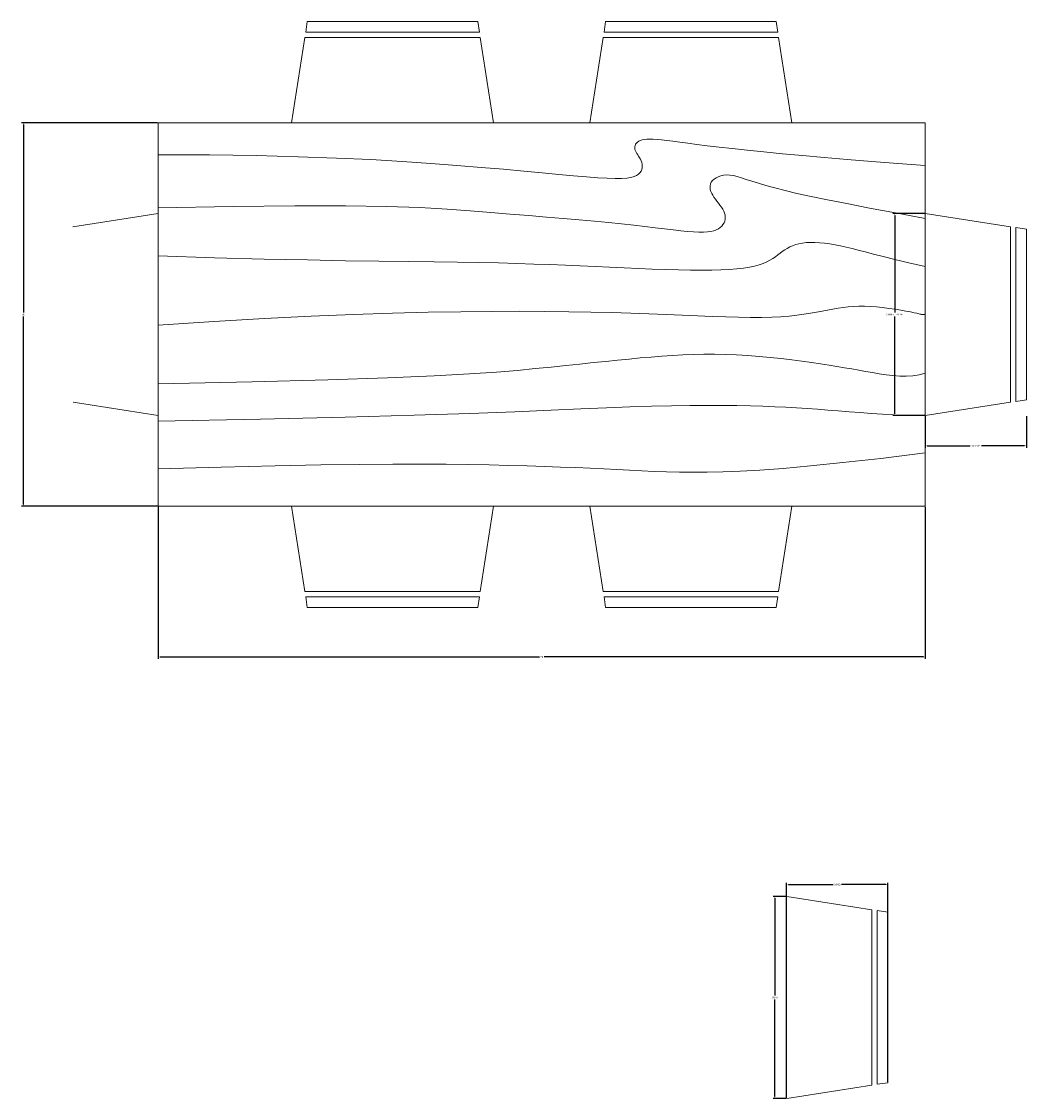
# Model space of a CAD drawing. Units: inches. Extents: x 821 to 2399, y 74 to 823.
# Tile 10 of 13: x 1930 to 2024, y 382 to 483. Entities that reach past the tile are written whole.
import ezdxf

# ---------------------------------------------------------------- set-up
doc = ezdxf.new("R2010")
doc.units = ezdxf.units.IN
doc.header["$MEASUREMENT"] = 0
doc.layers.get('0').update_dxf_attribs({"lineweight": 53})
doc.layers.add('A-ANNO-DIMS', color=2, linetype='Continuous', lineweight=18)
doc.layers.add('A-FURN', color=8, linetype='Continuous', lineweight=18)
doc.styles.get("Standard").update_dxf_attribs({"font": 'arial.ttf'})
doc.dimstyles.get("Standard").update_dxf_attribs({"dimtxt": 0.18, "dimasz": 0.18, "dimexe": 0.18, "dimexo": 0.0625, "dimgap": 0.09, "dimtad": 0, "dimtih": 1, "dimtoh": 1, "dimdec": 4, "dimzin": 0, "dimdsep": 46, "dimtxsty": 'Standard', "dimcen": 0.09, "dimadec": 0, "dimazin": 0, "dimtfac": 1, "dimtdec": 4, "dimtofl": 0, "dimtmove": 0, "dimatfit": 3, "dimfxl": 1, "dimtolj": 1, "dimtzin": 0, "dimarcsym": 0})

# ---------------------------------------------------------------- blocks, each defined once
blk = doc.blocks.new('CHAIR-DINING-19IN')
for p, q in [((1.48, 9.5), (1.33, 8.5)), ((1.48, 9.5), (17.48, 9.5)), ((17.64, 8.5), (17.48, 9.5)), ((17.64, 8.5), (1.33, 8.5)), ((1.25, 8), (0, 0)), ((1.25, 8), (17.72, 8)), ((18.97, 0), (17.72, 8))]:
    blk.add_line(p, q)
blk = doc.blocks.new('*D66')
at = {"layer": 'A-ANNO-DIMS', "color": 0, "lineweight": -2, "transparency": 16777216}
for p, q in [((2014.41, 464.93), (2011.44, 464.93)), ((2011.62, 464.75), (2011.62, 455.63)), ((2011.62, 446.14), (2011.62, 455.27)), ((2014.41, 445.96), (2011.44, 445.96))]:
    blk.add_line(p, q, dxfattribs=at)
at = {"layer": 'A-ANNO-DIMS', "color": 0, "lineweight": 50, "transparency": 16777216}
for points in [[(2011.59, 464.75), (2011.65, 464.75), (2011.62, 464.93)], [(2011.59, 446.14), (2011.65, 446.14), (2011.62, 445.96)]]:
    blk.add_solid(points, dxfattribs=at)
at = {"layer": 'Defpoints', "color": 0, "lineweight": 50, "transparency": 16777216}
for p in [(2014.47, 464.93), (2011.62, 445.96), (2014.47, 445.96)]:
    blk.add_point(p, dxfattribs=at)
at = {"layer": 'A-ANNO-DIMS', "color": 0, "transparency": 16777216, "insert": (2011.62, 455.45), "char_height": 0.18, "attachment_point": 5}
blk.add_mtext('\\A1;CHAIR 19 TYP.', dxfattribs=at)
blk = doc.blocks.new('*D67')
at = {"layer": 'A-ANNO-DIMS', "color": 0, "lineweight": -2, "transparency": 16777216}
for p, q in [((2014.47, 445.9), (2014.47, 442.94)), ((2023.97, 445.9), (2023.97, 442.94)), ((2014.65, 443.12), (2018.7, 443.12)), ((2023.79, 443.12), (2019.74, 443.12))]:
    blk.add_line(p, q, dxfattribs=at)
at = {"layer": 'A-ANNO-DIMS', "color": 0, "lineweight": 50, "transparency": 16777216}
for points in [[(2014.65, 443.15), (2014.65, 443.09), (2014.47, 443.12)], [(2023.79, 443.15), (2023.79, 443.09), (2023.97, 443.12)]]:
    blk.add_solid(points, dxfattribs=at)
at = {"layer": 'Defpoints', "color": 0, "lineweight": 50, "transparency": 16777216}
for p in [(2014.47, 445.96), (2023.97, 445.96), (2023.97, 443.12)]:
    blk.add_point(p, dxfattribs=at)
at = {"layer": 'A-ANNO-DIMS', "color": 0, "transparency": 16777216, "insert": (2019.22, 443.12), "char_height": 0.18, "attachment_point": 5}
blk.add_mtext('\\A1;10 TYP.', dxfattribs=at)
blk = doc.blocks.new('*D107')
at = {"layer": 'A-ANNO-DIMS', "color": 0, "lineweight": -2, "transparency": 16777216}
for p, q in [((1942.47, 437.39), (1942.47, 423.12)), ((2014.47, 437.39), (2014.47, 423.12)), ((1942.65, 423.3), (1978.25, 423.3)), ((2014.29, 423.3), (1978.69, 423.3))]:
    blk.add_line(p, q, dxfattribs=at)
at = {"layer": 'A-ANNO-DIMS', "color": 0, "lineweight": 50, "transparency": 16777216}
for points in [[(1942.65, 423.33), (1942.65, 423.27), (1942.47, 423.3)], [(2014.29, 423.33), (2014.29, 423.27), (2014.47, 423.3)]]:
    blk.add_solid(points, dxfattribs=at)
at = {"layer": 'Defpoints', "color": 0, "lineweight": 50, "transparency": 16777216}
for p in [(1942.47, 437.45), (2014.47, 437.45), (2014.47, 423.3)]:
    blk.add_point(p, dxfattribs=at)
at = {"layer": 'A-ANNO-DIMS', "color": 0, "transparency": 16777216, "insert": (1978.47, 423.3), "char_height": 0.18, "attachment_point": 5}
blk.add_mtext('\\A1;72', dxfattribs=at)
blk = doc.blocks.new('*D108')
at = {"layer": 'A-ANNO-DIMS', "color": 0, "lineweight": -2, "transparency": 16777216}
for p, q in [((1942.41, 473.45), (1929.64, 473.45)), ((1929.82, 473.27), (1929.82, 455.63)), ((1929.82, 437.63), (1929.82, 455.27)), ((1942.41, 437.45), (1929.64, 437.45))]:
    blk.add_line(p, q, dxfattribs=at)
at = {"layer": 'A-ANNO-DIMS', "color": 0, "lineweight": 50, "transparency": 16777216}
for points in [[(1929.79, 473.27), (1929.85, 473.27), (1929.82, 473.45)], [(1929.79, 437.63), (1929.85, 437.63), (1929.82, 437.45)]]:
    blk.add_solid(points, dxfattribs=at)
at = {"layer": 'Defpoints', "color": 0, "lineweight": 50, "transparency": 16777216}
for p in [(1929.82, 473.45), (1942.47, 473.45), (1942.47, 437.45)]:
    blk.add_point(p, dxfattribs=at)
at = {"layer": 'A-ANNO-DIMS', "color": 0, "transparency": 16777216, "insert": (1929.82, 455.45), "char_height": 0.18, "attachment_point": 5}
blk.add_mtext('\\A1;36', dxfattribs=at)
blk = doc.blocks.new('*D118')
at = {"layer": 'A-ANNO-DIMS', "color": 0, "lineweight": -2, "transparency": 16777216}
for p, q in [((2001.46, 381.92), (2001.46, 402.11)), ((2001.64, 401.93), (2005.82, 401.93)), ((2010.78, 401.93), (2006.61, 401.93)), ((2010.96, 383.41), (2010.96, 402.11))]:
    blk.add_line(p, q, dxfattribs=at)
at = {"layer": 'A-ANNO-DIMS', "color": 0, "lineweight": 50, "transparency": 16777216}
for points in [[(2001.64, 401.96), (2001.64, 401.9), (2001.46, 401.93)], [(2010.78, 401.96), (2010.78, 401.9), (2010.96, 401.93)]]:
    blk.add_solid(points, dxfattribs=at)
at = {"layer": 'Defpoints', "color": 0, "lineweight": 50, "transparency": 16777216}
for p in [(2010.96, 401.93), (2010.96, 383.34), (2001.46, 381.86)]:
    blk.add_point(p, dxfattribs=at)
at = {"layer": 'A-ANNO-DIMS', "color": 0, "transparency": 16777216, "insert": (2006.21, 401.93), "char_height": 0.18, "attachment_point": 5}
blk.add_mtext('\\A1;9.502', dxfattribs=at)
blk = doc.blocks.new('*D119')
at = {"layer": 'A-ANNO-DIMS', "color": 0, "lineweight": -2, "transparency": 16777216}
for p, q in [((2001.4, 400.83), (2000.18, 400.83)), ((2000.36, 400.65), (2000.36, 391.53)), ((2000.36, 382.04), (2000.36, 391.16)), ((2001.4, 381.86), (2000.18, 381.86))]:
    blk.add_line(p, q, dxfattribs=at)
at = {"layer": 'A-ANNO-DIMS', "color": 0, "lineweight": 50, "transparency": 16777216}
for points in [[(2000.33, 400.65), (2000.39, 400.65), (2000.36, 400.83)], [(2000.33, 382.04), (2000.39, 382.04), (2000.36, 381.86)]]:
    blk.add_solid(points, dxfattribs=at)
at = {"layer": 'Defpoints', "color": 0, "lineweight": 50, "transparency": 16777216}
for p in [(2000.36, 400.83), (2001.46, 400.83), (2001.46, 381.86)]:
    blk.add_point(p, dxfattribs=at)
at = {"layer": 'A-ANNO-DIMS', "color": 0, "transparency": 16777216, "insert": (2000.36, 391.34), "char_height": 0.18, "attachment_point": 5}
blk.add_mtext('\\A1;18.97', dxfattribs=at)

msp = doc.modelspace()

# ---------------------------------------------------------------- linework, layer by layer
at = {"layer": 'A-FURN'}
for p, q in [((2014.4703, 473.4496), (1942.4703, 473.4496)), ((1942.4703, 473.4496), (1942.4703, 437.4496)), ((2014.4703, 437.4496), (2014.4703, 473.4496)), ((1934.4697, 463.6839), (1942.4727, 464.9344)), ((1942.4727, 445.9649), (1934.471, 447.2151)), ((1942.4703, 437.4496), (2014.4703, 437.4496))]:
    msp.add_line(p, q, dxfattribs=at)
for points in [[(1942.4703, 470.4496), (1947.2931, 470.4272), (1951.6624, 470.3637), (1955.6165, 470.265), (1959.1943, 470.1371), (1962.4341, 469.9857), (1965.3746, 469.8168), (1968.0544, 469.6361), (1970.512, 469.4496), (1972.7799, 469.2628), (1974.8668, 469.0798), (1976.7749, 468.9047), (1978.5068, 468.7413), (1980.0648, 468.5935), (1981.4514, 468.4652), (1982.6691, 468.3604), (1983.7203, 468.2829), (1984.6096, 468.2357), (1985.3505, 468.2178), (1985.9586, 468.2273), (1986.4495, 468.2621), (1986.8388, 468.3204), (1987.1422, 468.4001), (1987.3752, 468.4994), (1987.5536, 468.6163), (1987.6908, 468.7486), (1987.7919, 468.8936), (1987.8598, 469.0484), (1987.8974, 469.21), (1987.9076, 469.3756), (1987.8935, 469.5421), (1987.8578, 469.7066), (1987.8036, 469.8663), (1987.7341, 470.0188), (1987.6539, 470.1645), (1987.5678, 470.3043), (1987.4807, 470.4392), (1987.3975, 470.5702), (1987.3232, 470.6983), (1987.2625, 470.8244), (1987.2203, 470.9496), (1987.2008, 471.0743), (1987.2047, 471.197), (1987.232, 471.3158), (1987.2828, 471.4288), (1987.357, 471.5339), (1987.4547, 471.6293), (1987.5758, 471.713), (1987.7203, 471.7829), (1987.8892, 471.8376), (1988.0875, 471.8767), (1988.3209, 471.9001), (1988.5953, 471.9079), (1988.9166, 471.9001), (1989.2906, 471.8767), (1989.7232, 471.8376), (1990.2203, 471.7829), (1990.7887, 471.7128), (1991.4397, 471.628), (1992.1854, 471.5295), (1993.038, 471.4184), (1994.0098, 471.2955), (1995.1129, 471.1619), (1996.3596, 471.0185), (1997.762, 470.8663), (1999.3293, 470.7063), (2001.0582, 470.5395), (2002.9424, 470.3668), (2004.9755, 470.1892), (2007.1512, 470.0077), (2009.4632, 469.8233), (2011.905, 469.6369), (2014.4703, 469.4496)], [(1942.4703, 465.4496), (1949.4937, 465.5924), (1955.2978, 465.654), (1960.0462, 465.6474), (1963.9026, 465.585), (1967.0304, 465.4797), (1969.5933, 465.3441), (1971.7549, 465.191), (1973.6786, 465.0329), (1975.5005, 464.8804), (1977.2457, 464.7348), (1978.9118, 464.595), (1980.4963, 464.46), (1981.9969, 464.329), (1983.4111, 464.2009), (1984.7363, 464.0748), (1985.9703, 463.9496), (1987.1114, 463.8251), (1988.1617, 463.7035), (1989.1241, 463.5878), (1990.0015, 463.4809), (1990.797, 463.3856), (1991.5133, 463.3051), (1992.1534, 463.2421), (1992.7203, 463.1996), (1993.2174, 463.1799), (1993.65, 463.1827), (1994.024, 463.2069), (1994.3453, 463.2517), (1994.6197, 463.316), (1994.8531, 463.3988), (1995.0514, 463.4993), (1995.2203, 463.6163), (1995.3647, 463.7488), (1995.4846, 463.8949), (1995.5792, 464.0528), (1995.6474, 464.2204), (1995.6883, 464.3959), (1995.7008, 464.5772), (1995.684, 464.7624), (1995.637, 464.9496), (1995.5598, 465.1371), (1995.4573, 465.3246), (1995.3352, 465.5121), (1995.1995, 465.6996), (1995.0559, 465.8871), (1994.9104, 466.0746), (1994.7688, 466.2621), (1994.637, 466.4496), (1994.5203, 466.6369), (1994.4221, 466.8233), (1994.3455, 467.0077), (1994.2932, 467.1892), (1994.2683, 467.3668), (1994.2737, 467.5395), (1994.3123, 467.7063), (1994.387, 467.8663), (1994.4998, 468.018), (1994.6487, 468.1579), (1994.8308, 468.2823), (1995.0432, 468.3871), (1995.283, 468.4685), (1995.5471, 468.5225), (1995.8328, 468.5453), (1996.137, 468.5329), (1996.4597, 468.4827), (1996.8121, 468.3969), (1997.2085, 468.2788), (1997.663, 468.1319), (1998.1898, 467.9596), (1998.803, 467.7654), (1999.5168, 467.5526), (2000.3453, 467.3246), (2001.306, 467.0832), (2002.4293, 466.8227), (2003.7489, 466.5358), (2005.2985, 466.2152), (2007.1117, 465.8537), (2009.2223, 465.4438), (2011.6639, 464.9782), (2014.4703, 464.4496)], [(1942.4703, 460.9496), (1947.7546, 460.7844), (1952.4013, 460.6592), (1956.4757, 460.5673), (1960.0432, 460.5017), (1963.1694, 460.4556), (1965.9195, 460.4223), (1968.3591, 460.3948), (1970.5536, 460.3663), (1972.5613, 460.3313), (1974.4117, 460.2895), (1976.1274, 460.2418), (1977.7307, 460.1892), (1979.2442, 460.1327), (1980.6903, 460.0733), (1982.0916, 460.0119), (1983.4703, 459.9496), (1984.8433, 459.8874), (1986.2047, 459.8272), (1987.5426, 459.7709), (1988.8453, 459.7204), (1990.1012, 459.6778), (1991.2984, 459.6449), (1992.4254, 459.6238), (1993.4703, 459.6163), (1994.4243, 459.6241), (1995.2893, 459.6475), (1996.0704, 459.6866), (1996.7724, 459.7413), (1997.4002, 459.8116), (1997.9586, 459.8975), (1998.4526, 459.9991), (1998.887, 460.1163), (1999.2672, 460.2486), (1999.6005, 460.3936), (1999.8948, 460.5484), (2000.1578, 460.71), (2000.3974, 460.8756), (2000.6214, 461.0421), (2000.8375, 461.2066), (2001.0537, 461.3663), (2001.2768, 461.5183), (2001.5107, 461.6605), (2001.7582, 461.7911), (2002.0224, 461.9079), (2002.3061, 462.0092), (2002.6123, 462.0928), (2002.9438, 462.157), (2003.3037, 462.1996), (2003.6938, 462.2193), (2004.1123, 462.2165), (2004.5561, 462.1923), (2005.0224, 462.1475), (2005.5082, 462.0832), (2006.0107, 462.0004), (2006.5268, 461.9), (2007.0537, 461.7829), (2007.5945, 461.6495), (2008.1774, 461.4965), (2008.8364, 461.3201), (2009.6057, 461.1163), (2010.5196, 460.8813), (2011.6123, 460.6111), (2012.9178, 460.3018), (2014.4703, 459.9496)], [(1942.4703, 454.4496), (1947.6788, 454.7905), (1952.4508, 455.0675), (1956.8184, 455.2868), (1960.814, 455.4548), (1964.4698, 455.5779), (1967.818, 455.6625), (1970.8907, 455.7148), (1973.7203, 455.7413), (1976.3363, 455.7475), (1978.7581, 455.7367), (1981.002, 455.7112), (1983.0849, 455.6736), (1985.0232, 455.6261), (1986.8336, 455.5714), (1988.5326, 455.5117), (1990.137, 455.4496), (1991.6602, 455.3876), (1993.1044, 455.3285), (1994.4685, 455.2753), (1995.7516, 455.2309), (1996.9526, 455.1981), (1998.0706, 455.1801), (1999.1046, 455.1796), (2000.0537, 455.1996), (2000.9184, 455.2419), (2001.706, 455.3038), (2002.4252, 455.3813), (2003.0849, 455.4704), (2003.6938, 455.5675), (2004.2607, 455.6684), (2004.7944, 455.7693), (2005.3037, 455.8663), (2005.7968, 455.9558), (2006.2802, 456.0355), (2006.7597, 456.1036), (2007.2412, 456.1579), (2007.7304, 456.1967), (2008.2333, 456.2178), (2008.7558, 456.2195), (2009.3037, 456.1996), (2009.8791, 456.1575), (2010.4697, 456.0967), (2011.0593, 456.0224), (2011.6318, 455.9392), (2012.1711, 455.8521), (2012.6611, 455.766), (2013.0856, 455.6858), (2013.4287, 455.6163), (2013.6802, 455.5613), (2013.8551, 455.5199), (2013.9743, 455.4903), (2014.0589, 455.4704), (2014.1297, 455.4584), (2014.208, 455.4522), (2014.3145, 455.4499), (2014.4703, 455.4496)], [(1942.4703, 448.9496), (1951.286, 449.1369), (1958.3863, 449.3233), (1964.0013, 449.5077), (1968.3609, 449.6892), (1971.6951, 449.8668), (1974.234, 450.0395), (1976.2074, 450.2063), (1977.8453, 450.3663), (1979.3411, 450.5186), (1980.7418, 450.6632), (1982.0575, 450.7999), (1983.2984, 450.9288), (1984.4749, 451.0499), (1985.5973, 451.1632), (1986.6756, 451.2686), (1987.7203, 451.3663), (1988.7408, 451.4558), (1989.7437, 451.5355), (1990.735, 451.6036), (1991.7203, 451.6579), (1992.7057, 451.6967), (1993.6969, 451.7178), (1994.6998, 451.7195), (1995.7203, 451.6996), (1996.7615, 451.6571), (1997.8154, 451.5941), (1998.8712, 451.5136), (1999.9182, 451.4184), (2000.9457, 451.3114), (2001.943, 451.1957), (2002.8992, 451.0741), (2003.8037, 450.9496), (2004.6488, 450.8247), (2005.4397, 450.7003), (2006.1848, 450.5768), (2006.8922, 450.4548), (2007.5703, 450.3348), (2008.2275, 450.2172), (2008.8719, 450.1025), (2009.512, 449.9913), (2010.154, 449.8852), (2010.7965, 449.7914), (2011.4361, 449.7181), (2012.0693, 449.6736), (2012.6927, 449.6662), (2013.303, 449.7042), (2013.8967, 449.7959), (2014.4703, 449.9496)], [(1942.4703, 445.4496), (1952.0681, 445.6366), (1960.0028, 445.8207), (1966.4864, 445.9989), (1971.7307, 446.1684), (1975.9477, 446.3261), (1979.3492, 446.4691), (1982.1472, 446.5946), (1984.5536, 446.6996), (1986.747, 446.782), (1988.7724, 446.8428), (1990.6415, 446.8842), (1992.3661, 446.9079), (1993.9579, 446.9161), (1995.4286, 446.9105), (1996.79, 446.8933), (1998.0537, 446.8663), (1999.2319, 446.8312), (2000.3388, 446.7888), (2001.3891, 446.7396), (2002.3974, 446.684), (2003.3784, 446.6225), (2004.3466, 446.5557), (2005.3168, 446.484), (2006.3037, 446.4079), (2007.3177, 446.3284), (2008.3531, 446.2484), (2009.4003, 446.1714), (2010.4495, 446.1007), (2011.4908, 446.0397), (2012.5146, 445.9919), (2013.511, 445.9608), (2014.4703, 445.9496)], [(1942.4703, 440.9496), (1948.3822, 441.1145), (1953.4371, 441.2374), (1957.7391, 441.3231), (1961.3922, 441.3767), (1964.5003, 441.4029), (1967.1676, 441.4066), (1969.4979, 441.3928), (1971.5953, 441.3663), (1973.5479, 441.3313), (1975.3798, 441.2895), (1977.0994, 441.2418), (1978.7151, 441.1892), (1980.235, 441.1327), (1981.6676, 441.0733), (1983.021, 441.0119), (1984.3036, 440.9496), (1985.5257, 440.8875), (1986.7053, 440.8279), (1987.8625, 440.7731), (1989.0172, 440.7257), (1990.1895, 440.688), (1991.3993, 440.6625), (1992.6668, 440.6517), (1994.012, 440.6579), (1995.4636, 440.6854), (1997.0855, 440.7445), (1998.9507, 440.8476), (2001.1318, 441.0069), (2003.7015, 441.2345), (2006.7327, 441.5427), (2010.298, 441.9437), (2014.4703, 442.4496)]]:
    msp.add_lwpolyline(points, dxfattribs=at)

# ---------------------------------------------------------------- block references
for p in [(1954.986, 473.447), (1982.986, 473.447)]:
    msp.add_blockref('CHAIR-DINING-19IN', p, dxfattribs=at)
at = {"layer": 'A-FURN', "rotation": 269.9999986166246}
msp.add_blockref('CHAIR-DINING-19IN', (2014.4677, 464.9339), dxfattribs=at)
at = {"layer": 'A-FURN', "extrusion": (0, 0, -1), "zscale": -1}
for p, rotation in [((-1954.986, 437.4522), 180.0000160409505), ((-1982.986, 437.4522), 180.0000160409505), ((-2001.4618, 381.8602), 90.00001604246143)]:
    msp.add_blockref('CHAIR-DINING-19IN', p, dxfattribs=dict(at, rotation=rotation))

# ---------------------------------------------------------------- dimensions: what is measured, and where the dimension line sits
at = {"layer": 'A-ANNO-DIMS'}
for base, p1, p2, override, picture, middle in [((1929.8197, 473.4496), (1942.4703, 437.4496), (1942.4703, 473.4496), {"dimdec": 0, "dimlfac": 1, "dimrnd": 0, "dimzin": 0, "dimdsep": 46, "dimlunit": 2}, '*D108', (1929.8197, 455.4496)), ((2000.362, 400.8293), (2001.462, 381.8598), (2001.462, 400.8293), {"dimdec": 2, "dimlfac": 1, "dimrnd": 0, "dimzin": 0, "dimdsep": 46, "dimlunit": 2}, '*D119', (2000.362, 391.3446))]:
    dim = msp.add_linear_dim(base=base, p1=p1, p2=p2, angle=90, dimstyle='Standard', override=override, dxfattribs=at)
    dim.commit()
    dim.dimension.update_dxf_attribs({"geometry": picture, "text_midpoint": middle})
for base, p1, p2, angle, text, picture, middle in [((2011.6225, 445.9648), (2014.4679, 464.9343), (2014.4679, 445.9648), 269.999999, 'CHAIR <> TYP.', '*D66', (2011.6225, 455.4496)), ((2023.9703, 443.1194), (2014.4679, 445.9648), (2023.9703, 445.9648), 359.999999, '<> TYP.', '*D67', (2019.2191, 443.1194))]:
    dim = msp.add_linear_dim(base=base, p1=p1, p2=p2, angle=angle, text=text, dimstyle='Standard', override={"dimdec": 0, "dimlfac": 1, "dimrnd": 0, "dimzin": 0, "dimdsep": 46, "dimlunit": 2}, dxfattribs=at)
    dim.commit()
    dim.dimension.update_dxf_attribs({"geometry": picture, "text_midpoint": middle})
for base, p1, p2, override, picture, middle in [((2014.4703, 423.2996), (1942.4703, 437.4496), (2014.4703, 437.4496), {"dimdec": 0, "dimlfac": 1, "dimrnd": 0, "dimzin": 0, "dimdsep": 46, "dimlunit": 2}, '*D107', (1978.4703, 423.2996)), ((2010.9644, 401.9293), (2001.462, 381.8598), (2010.9644, 383.3445), {"dimdec": 3, "dimlfac": 1, "dimrnd": 0, "dimzin": 0, "dimdsep": 46, "dimlunit": 2}, '*D118', (2006.2132, 401.9293))]:
    dim = msp.add_linear_dim(base=base, p1=p1, p2=p2, dimstyle='Standard', override=override, dxfattribs=at)
    dim.commit()
    dim.dimension.update_dxf_attribs({"geometry": picture, "text_midpoint": middle})

doc.saveas('drawing.dxf')
